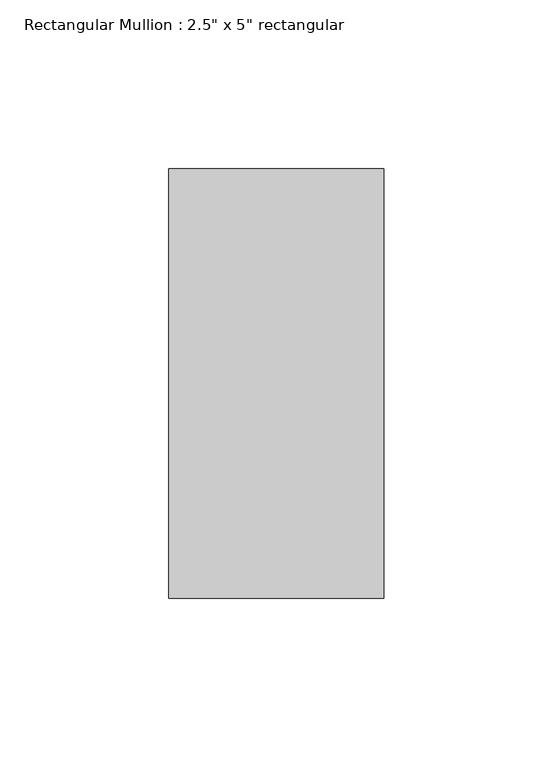
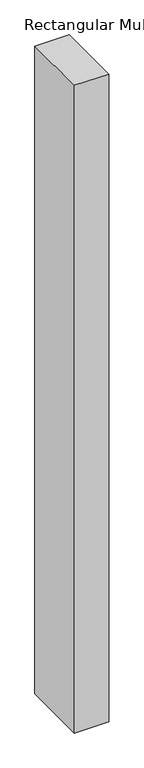
"""IFC4 building model written with IfcOpenShell, lengths in millimetres: member geometry."""

from ifc_helpers import new_model, si_unit, frame, origin, place, context, project, spatial, polyline, outline, extrude, source, transform, mapped, element, save


def member_e78f2157(model_context):
    return source(origin(), model_context, "Body", "SweptSolid", [
        extrude(outline(polyline([(0.0, 63.5), (0.0, -63.5), (-63.5, -63.5), (-63.5, 63.5), (0.0, 63.5)])), frame((0.0, 0.0, -1270.9564694), z_axis=(0.0, 0.0, 1.0), x_axis=(1.0, 0.0, 0.0)), (0.0, 0.0, 1.0), 1270.9564694),
    ])


if __name__ == "__main__":
    model = new_model("IFC4")
    model_context = context("Model", 3, world=origin())
    ifc_project = project(units=[si_unit("LENGTHUNIT", "METRE", prefix="MILLI")], contexts=[model_context])
    site = spatial("IfcSite", under=ifc_project)
    building = spatial("IfcBuilding", under=site)
    placement = place(None, origin())
    member_shape = member_e78f2157(model_context)
    element("IfcMember", 1, ObjectType="Rectangular Mullion : 2.5\" x 5\" rectangular", at=placement, inside=building, context=model_context, shape_type="MappedRepresentation", body=[
        mapped(member_shape, transform((0.0, 0.0, 0.0), x_axis=(1.0, 0.0, 0.0), y_axis=(0.0, 1.0, 0.0), z_axis=(0.0, 0.0, 1.0))),
    ])
    save(model, "model.ifc")

# Revit data of these elements
# Type "Rectangular Mullion : 2.5\" x 5\" rectangular"
#   built-in parameter 1007304 = 0.416667 (stored number, unit not read)
#   built-in parameter 1007301 = 0.104167 (stored number, unit not read)
#   built-in parameter 1007300 = 0.104167 (stored number, unit not read)
# Element 1 (IfcMember, "Rectangular Mullion : 2.5\" x 5\" rectangular")
#   Materials on its faces: "Aluminum"
# Materials
#   "Aluminum": class "Metal", colour RGB 247 247 247, transparency 0, Description = "Aluminum 6061", Cost = 0
